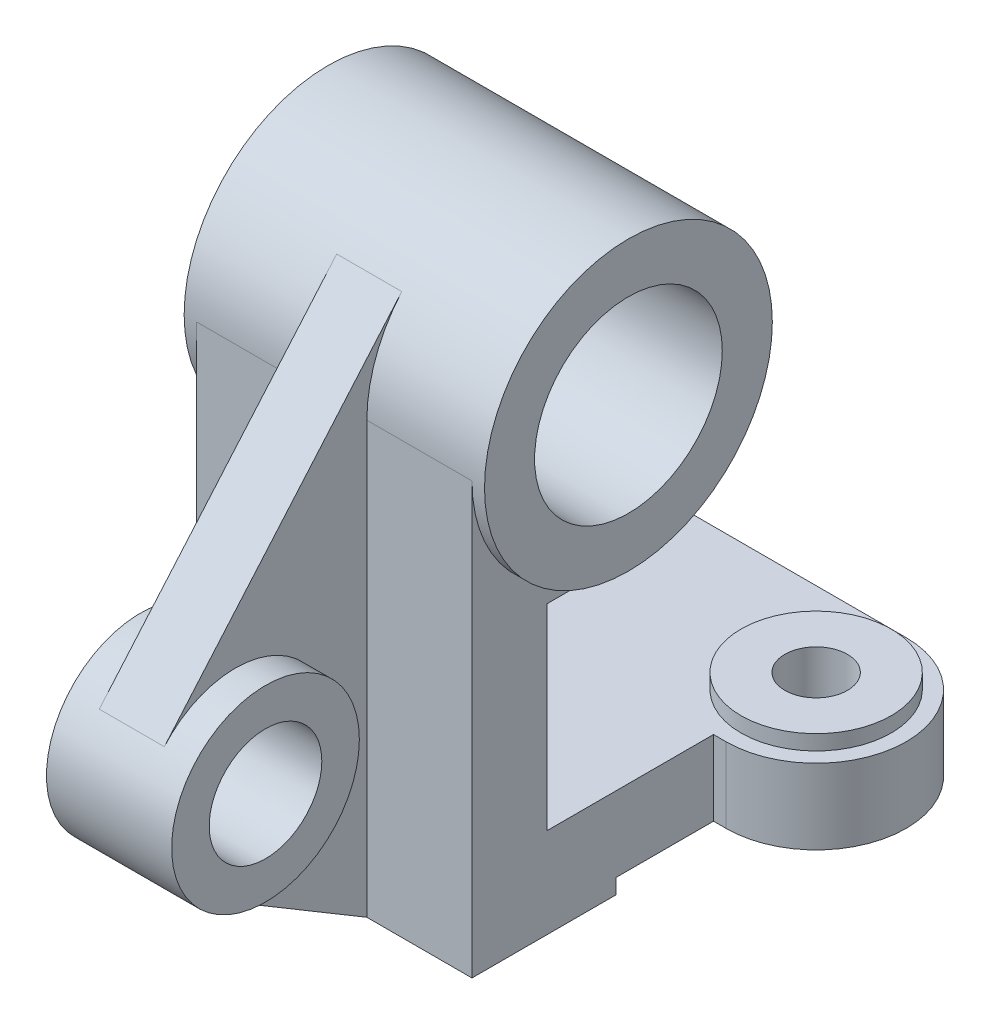
ISO-10303-21;
HEADER;
FILE_DESCRIPTION(('STEP AP214'),'2;1');
FILE_NAME('part.step','',(''),(''),'','','');
FILE_SCHEMA(('AUTOMOTIVE_DESIGN { 1 0 10303 214 1 1 1 1 }'));
ENDSEC;
DATA;
#1=APPLICATION_CONTEXT('core data for automotive mechanical design processes');
#2=APPLICATION_PROTOCOL_DEFINITION('international standard','automotive_design',2000,#1);
#3=PRODUCT_CONTEXT('',#1,'mechanical');
#4=PRODUCT('Part','Part','',(#3));
#5=PRODUCT_RELATED_PRODUCT_CATEGORY('part','',(#4));
#6=PRODUCT_DEFINITION_FORMATION('','',#4);
#7=PRODUCT_DEFINITION_CONTEXT('part definition',#1,'design');
#8=PRODUCT_DEFINITION('design','',#6,#7);
#9=PRODUCT_DEFINITION_SHAPE('','',#8);
#10=(LENGTH_UNIT() NAMED_UNIT(*) SI_UNIT(.MILLI.,.METRE.));
#11=(NAMED_UNIT(*) PLANE_ANGLE_UNIT() SI_UNIT($,.RADIAN.));
#12=(NAMED_UNIT(*) SI_UNIT($,.STERADIAN.) SOLID_ANGLE_UNIT());
#13=UNCERTAINTY_MEASURE_WITH_UNIT(LENGTH_MEASURE(1.E-05),#10,'distance_accuracy_value','');
#14=(GEOMETRIC_REPRESENTATION_CONTEXT(3) GLOBAL_UNCERTAINTY_ASSIGNED_CONTEXT((#13)) GLOBAL_UNIT_ASSIGNED_CONTEXT((#10,
#11,#12)) REPRESENTATION_CONTEXT('',''));
#15=CARTESIAN_POINT('',(0.,0.,0.));
#16=DIRECTION('',(0.,0.,1.));
#17=DIRECTION('',(1.,0.,0.));
#18=AXIS2_PLACEMENT_3D('',#15,#16,#17);
#19=CARTESIAN_POINT('',(55.,0.,57.5));
#20=DIRECTION('',(0.,0.,-1.));
#21=DIRECTION('',(0.,1.,0.));
#22=AXIS2_PLACEMENT_3D('',#19,#20,#21);
#23=PLANE('',#22);
#24=DIRECTION('',(0.,1.,0.));
#25=VECTOR('',#24,1.);
#26=CARTESIAN_POINT('',(-13.,-172.,57.5));
#27=LINE('',#26,#25);
#28=CARTESIAN_POINT('',(-13.,-172.,57.5));
#29=VERTEX_POINT('',#28);
#30=CARTESIAN_POINT('',(-13.,0.,57.5));
#31=VERTEX_POINT('',#30);
#32=EDGE_CURVE('E53',#29,#31,#27,.T.);
#33=ORIENTED_EDGE('',*,*,#32,.T.);
#34=DIRECTION('',(-1.,0.,0.));
#35=VECTOR('',#34,1.);
#36=CARTESIAN_POINT('',(55.,0.,57.5));
#37=LINE('',#36,#35);
#38=CARTESIAN_POINT('',(-55.,0.,57.5));
#39=VERTEX_POINT('',#38);
#40=EDGE_CURVE('E61',#31,#39,#37,.T.);
#41=ORIENTED_EDGE('',*,*,#40,.T.);
#42=DIRECTION('',(0.,-1.,0.));
#43=VECTOR('',#42,1.);
#44=CARTESIAN_POINT('',(-55.,0.,57.5));
#45=LINE('',#44,#43);
#46=CARTESIAN_POINT('',(-55.,-172.,57.5));
#47=VERTEX_POINT('',#46);
#48=EDGE_CURVE('E287',#39,#47,#45,.T.);
#49=ORIENTED_EDGE('',*,*,#48,.T.);
#50=DIRECTION('',(-1.,0.,0.));
#51=VECTOR('',#50,1.);
#52=CARTESIAN_POINT('',(55.,-172.,57.5));
#53=LINE('',#52,#51);
#54=EDGE_CURVE('E319',#29,#47,#53,.T.);
#55=ORIENTED_EDGE('',*,*,#54,.F.);
#56=EDGE_LOOP('',(#33,#41,#49,#55));
#57=FACE_BOUND('',#56,.T.);
#58=ADVANCED_FACE('F39',(#57),#23,.F.);
#59=CARTESIAN_POINT('',(-60.,0.,0.));
#60=DIRECTION('',(1.,0.,0.));
#61=DIRECTION('',(0.,0.,-1.));
#62=AXIS2_PLACEMENT_3D('',#59,#60,#61);
#63=CYLINDRICAL_SURFACE('',#62,57.5);
#64=CARTESIAN_POINT('',(13.,0.,0.));
#65=DIRECTION('',(-1.,0.,0.));
#66=DIRECTION('',(0.,0.,-1.));
#67=AXIS2_PLACEMENT_3D('',#64,#65,#66);
#68=CIRCLE('',#67,57.5);
#69=CARTESIAN_POINT('',(13.,0.,57.5));
#70=VERTEX_POINT('',#69);
#71=CARTESIAN_POINT('',(13.,37.5380186304021,43.5562527922637));
#72=VERTEX_POINT('',#71);
#73=EDGE_CURVE('E360',#70,#72,#68,.T.);
#74=ORIENTED_EDGE('',*,*,#73,.F.);
#75=CARTESIAN_POINT('',(55.,0.,57.5));
#76=VERTEX_POINT('',#75);
#77=EDGE_CURVE('E322',#76,#70,#37,.T.);
#78=ORIENTED_EDGE('',*,*,#77,.F.);
#79=CARTESIAN_POINT('',(55.,0.,0.));
#80=DIRECTION('',(-1.,0.,0.));
#81=DIRECTION('',(0.,0.,-1.));
#82=AXIS2_PLACEMENT_3D('',#79,#80,#81);
#83=CIRCLE('',#82,57.5);
#84=CARTESIAN_POINT('',(55.,-57.5,0.));
#85=VERTEX_POINT('',#84);
#86=EDGE_CURVE('E270',#85,#76,#83,.T.);
#87=ORIENTED_EDGE('',*,*,#86,.F.);
#88=DIRECTION('',(-1.,0.,0.));
#89=VECTOR('',#88,1.);
#90=CARTESIAN_POINT('',(55.,-57.5,0.));
#91=LINE('',#90,#89);
#92=CARTESIAN_POINT('',(-55.,-57.5,0.));
#93=VERTEX_POINT('',#92);
#94=EDGE_CURVE('E286',#85,#93,#91,.T.);
#95=ORIENTED_EDGE('',*,*,#94,.T.);
#96=CARTESIAN_POINT('',(-55.,0.,0.));
#97=DIRECTION('',(-1.,0.,0.));
#98=DIRECTION('',(0.,0.,-1.));
#99=AXIS2_PLACEMENT_3D('',#96,#97,#98);
#100=CIRCLE('',#99,57.5);
#101=EDGE_CURVE('E227',#93,#39,#100,.T.);
#102=ORIENTED_EDGE('',*,*,#101,.T.);
#103=ORIENTED_EDGE('',*,*,#40,.F.);
#104=CARTESIAN_POINT('',(-13.,0.,0.));
#105=DIRECTION('',(-1.,0.,0.));
#106=DIRECTION('',(0.,0.,-1.));
#107=AXIS2_PLACEMENT_3D('',#104,#105,#106);
#108=CIRCLE('',#107,57.5);
#109=CARTESIAN_POINT('',(-13.,37.5380186304021,43.5562527922637));
#110=VERTEX_POINT('',#109);
#111=EDGE_CURVE('E196',#31,#110,#108,.T.);
#112=ORIENTED_EDGE('',*,*,#111,.T.);
#113=DIRECTION('',(-1.,0.,0.));
#114=VECTOR('',#113,1.);
#115=CARTESIAN_POINT('',(13.,37.5380186304021,43.5562527922637));
#116=LINE('',#115,#114);
#117=EDGE_CURVE('E202',#72,#110,#116,.T.);
#118=ORIENTED_EDGE('',*,*,#117,.F.);
#119=EDGE_LOOP('',(#74,#78,#87,#95,#102,#103,#112,#118));
#120=FACE_BOUND('',#119,.T.);
#121=CARTESIAN_POINT('',(-60.,0.,0.));
#122=DIRECTION('',(1.,0.,0.));
#123=DIRECTION('',(0.,0.,-1.));
#124=AXIS2_PLACEMENT_3D('',#121,#122,#123);
#125=CIRCLE('',#124,57.5);
#126=CARTESIAN_POINT('',(-60.,0.,-57.5));
#127=VERTEX_POINT('',#126);
#128=EDGE_CURVE('E11',#127,#127,#125,.T.);
#129=ORIENTED_EDGE('',*,*,#128,.T.);
#130=EDGE_LOOP('',(#129));
#131=FACE_BOUND('',#130,.T.);
#132=CARTESIAN_POINT('',(60.,0.,0.));
#133=DIRECTION('',(1.,0.,0.));
#134=DIRECTION('',(0.,0.,-1.));
#135=AXIS2_PLACEMENT_3D('',#132,#133,#134);
#136=CIRCLE('',#135,57.5);
#137=CARTESIAN_POINT('',(60.,0.,-57.5));
#138=VERTEX_POINT('',#137);
#139=EDGE_CURVE('E43',#138,#138,#136,.T.);
#140=ORIENTED_EDGE('',*,*,#139,.F.);
#141=EDGE_LOOP('',(#140));
#142=FACE_BOUND('',#141,.T.);
#143=ADVANCED_FACE('F41',(#120,#131,#142),#63,.T.);
#144=CARTESIAN_POINT('',(-60.,0.,0.));
#145=DIRECTION('',(1.,0.,0.));
#146=DIRECTION('',(0.,0.,-1.));
#147=AXIS2_PLACEMENT_3D('',#144,#145,#146);
#148=PLANE('',#147);
#149=CARTESIAN_POINT('',(-60.,0.,0.));
#150=DIRECTION('',(1.,0.,0.));
#151=DIRECTION('',(0.,0.,-1.));
#152=AXIS2_PLACEMENT_3D('',#149,#150,#151);
#153=CIRCLE('',#152,37.5);
#154=CARTESIAN_POINT('',(-60.,0.,-37.5));
#155=VERTEX_POINT('',#154);
#156=EDGE_CURVE('E327',#155,#155,#153,.T.);
#157=ORIENTED_EDGE('',*,*,#156,.T.);
#158=EDGE_LOOP('',(#157));
#159=FACE_BOUND('',#158,.T.);
#160=ORIENTED_EDGE('',*,*,#128,.F.);
#161=EDGE_LOOP('',(#160));
#162=FACE_BOUND('',#161,.T.);
#163=ADVANCED_FACE('F338',(#159,#162),#148,.F.);
#164=CARTESIAN_POINT('',(60.,0.,0.));
#165=DIRECTION('',(1.,0.,0.));
#166=DIRECTION('',(0.,0.,-1.));
#167=AXIS2_PLACEMENT_3D('',#164,#165,#166);
#168=PLANE('',#167);
#169=CARTESIAN_POINT('',(60.,0.,0.));
#170=DIRECTION('',(1.,0.,0.));
#171=DIRECTION('',(0.,0.,-1.));
#172=AXIS2_PLACEMENT_3D('',#169,#170,#171);
#173=CIRCLE('',#172,37.5);
#174=CARTESIAN_POINT('',(60.,0.,-37.5));
#175=VERTEX_POINT('',#174);
#176=EDGE_CURVE('E330',#175,#175,#173,.T.);
#177=ORIENTED_EDGE('',*,*,#176,.F.);
#178=EDGE_LOOP('',(#177));
#179=FACE_BOUND('',#178,.T.);
#180=ORIENTED_EDGE('',*,*,#139,.T.);
#181=EDGE_LOOP('',(#180));
#182=FACE_BOUND('',#181,.T.);
#183=ADVANCED_FACE('F336',(#179,#182),#168,.T.);
#184=CARTESIAN_POINT('',(-60.,0.,0.));
#185=DIRECTION('',(1.,0.,0.));
#186=DIRECTION('',(0.,0.,-1.));
#187=AXIS2_PLACEMENT_3D('',#184,#185,#186);
#188=CYLINDRICAL_SURFACE('',#187,37.5);
#189=CARTESIAN_POINT('',(-60.,0.,-37.5));
#190=CARTESIAN_POINT('',(-58.75,0.,-37.5));
#191=CARTESIAN_POINT('',(-57.5,0.,-37.5));
#192=CARTESIAN_POINT('',(-55.,0.,-37.5));
#193=CARTESIAN_POINT('',(-53.75,0.,-37.5));
#194=CARTESIAN_POINT('',(-51.25,0.,-37.5));
#195=CARTESIAN_POINT('',(-50.,0.,-37.5));
#196=CARTESIAN_POINT('',(-47.5,0.,-37.5));
#197=CARTESIAN_POINT('',(-46.25,0.,-37.5));
#198=CARTESIAN_POINT('',(-43.75,0.,-37.5));
#199=CARTESIAN_POINT('',(-42.5,0.,-37.5));
#200=CARTESIAN_POINT('',(-40.,0.,-37.5));
#201=CARTESIAN_POINT('',(-38.75,0.,-37.5));
#202=CARTESIAN_POINT('',(-36.25,0.,-37.5));
#203=CARTESIAN_POINT('',(-35.,0.,-37.5));
#204=CARTESIAN_POINT('',(-32.5,0.,-37.5));
#205=CARTESIAN_POINT('',(-31.25,0.,-37.5));
#206=CARTESIAN_POINT('',(-28.75,0.,-37.5));
#207=CARTESIAN_POINT('',(-27.5,0.,-37.5));
#208=CARTESIAN_POINT('',(-25.,0.,-37.5));
#209=CARTESIAN_POINT('',(-23.75,0.,-37.5));
#210=CARTESIAN_POINT('',(-21.25,0.,-37.5));
#211=CARTESIAN_POINT('',(-20.,0.,-37.5));
#212=CARTESIAN_POINT('',(-17.5,0.,-37.5));
#213=CARTESIAN_POINT('',(-16.25,0.,-37.5));
#214=CARTESIAN_POINT('',(-13.75,0.,-37.5));
#215=CARTESIAN_POINT('',(-12.5,0.,-37.5));
#216=CARTESIAN_POINT('',(-10.,0.,-37.5));
#217=CARTESIAN_POINT('',(-8.75000000000001,0.,-37.5));
#218=CARTESIAN_POINT('',(-6.25000000000001,0.,-37.5));
#219=CARTESIAN_POINT('',(-5.00000000000001,0.,-37.5));
#220=CARTESIAN_POINT('',(-2.50000000000001,0.,-37.5));
#221=CARTESIAN_POINT('',(-1.25000000000001,0.,-37.5));
#222=CARTESIAN_POINT('',(1.24999999999999,0.,-37.5));
#223=CARTESIAN_POINT('',(2.5,0.,-37.5));
#224=CARTESIAN_POINT('',(5.,0.,-37.5));
#225=CARTESIAN_POINT('',(6.25,0.,-37.5));
#226=CARTESIAN_POINT('',(8.75,0.,-37.5));
#227=CARTESIAN_POINT('',(9.99999999999999,0.,-37.5));
#228=CARTESIAN_POINT('',(12.5,0.,-37.5));
#229=CARTESIAN_POINT('',(13.75,0.,-37.5));
#230=CARTESIAN_POINT('',(16.25,0.,-37.5));
#231=CARTESIAN_POINT('',(17.5,0.,-37.5));
#232=CARTESIAN_POINT('',(20.,0.,-37.5));
#233=CARTESIAN_POINT('',(21.25,0.,-37.5));
#234=CARTESIAN_POINT('',(23.75,0.,-37.5));
#235=CARTESIAN_POINT('',(25.,0.,-37.5));
#236=CARTESIAN_POINT('',(27.5,0.,-37.5));
#237=CARTESIAN_POINT('',(28.75,0.,-37.5));
#238=CARTESIAN_POINT('',(31.25,0.,-37.5));
#239=CARTESIAN_POINT('',(32.5,0.,-37.5));
#240=CARTESIAN_POINT('',(35.,0.,-37.5));
#241=CARTESIAN_POINT('',(36.25,0.,-37.5));
#242=CARTESIAN_POINT('',(38.75,0.,-37.5));
#243=CARTESIAN_POINT('',(40.,0.,-37.5));
#244=CARTESIAN_POINT('',(42.5,0.,-37.5));
#245=CARTESIAN_POINT('',(43.75,0.,-37.5));
#246=CARTESIAN_POINT('',(46.25,0.,-37.5));
#247=CARTESIAN_POINT('',(47.5,0.,-37.5));
#248=CARTESIAN_POINT('',(50.,0.,-37.5));
#249=CARTESIAN_POINT('',(51.25,0.,-37.5));
#250=CARTESIAN_POINT('',(53.75,0.,-37.5));
#251=CARTESIAN_POINT('',(55.,0.,-37.5));
#252=CARTESIAN_POINT('',(57.5,0.,-37.5));
#253=CARTESIAN_POINT('',(58.75,0.,-37.5));
#254=CARTESIAN_POINT('',(60.,0.,-37.5));
#255=B_SPLINE_CURVE_WITH_KNOTS('',3,(#189,#190,#191,#192,#193,#194,#195,#196,#197,#198,#199,
#200,#201,#202,#203,#204,#205,#206,#207,#208,#209,#210,#211,#212,#213,#214,#215,#216,#217,#218,
#219,#220,#221,#222,#223,#224,#225,#226,#227,#228,#229,#230,#231,#232,#233,#234,#235,#236,#237,
#238,#239,#240,#241,#242,#243,#244,#245,#246,#247,#248,#249,#250,#251,#252,#253,#254),
.UNSPECIFIED.,.F.,.F.,(4,2,2,2,2,2,2,2,2,2,2,2,2,2,2,2,2,2,2,2,2,2,2,2,2,2,2,2,2,2,2,2,4),(0.,
3.75,7.5,11.25,15.,18.75,22.5,26.25,30.,33.75,37.5,41.25,45.,48.75,52.5,56.25,60.,63.75,67.5,
71.25,75.,78.75,82.5,86.25,90.,93.75,97.5,101.25,105.,108.75,112.5,116.25,120.),.UNSPECIFIED.);
#256=EDGE_CURVE('BSEAM331',#155,#175,#255,.T.);
#257=ORIENTED_EDGE('',*,*,#156,.F.);
#258=ORIENTED_EDGE('',*,*,#176,.T.);
#259=ORIENTED_EDGE('',*,*,#256,.T.);
#260=ORIENTED_EDGE('',*,*,#256,.F.);
#261=EDGE_LOOP('',(#257,#259,#258,#260));
#262=FACE_BOUND('',#261,.T.);
#263=ADVANCED_FACE('F331',(#262),#188,.F.);
#264=ORIENTED_EDGE('',*,*,#77,.T.);
#265=DIRECTION('',(0.,1.,0.));
#266=VECTOR('',#265,1.);
#267=CARTESIAN_POINT('',(13.,-172.,57.5));
#268=LINE('',#267,#266);
#269=CARTESIAN_POINT('',(13.,-172.,57.5));
#270=VERTEX_POINT('',#269);
#271=EDGE_CURVE('E365',#270,#70,#268,.T.);
#272=ORIENTED_EDGE('',*,*,#271,.F.);
#273=CARTESIAN_POINT('',(55.,-172.,57.5));
#274=VERTEX_POINT('',#273);
#275=EDGE_CURVE('E321',#274,#270,#53,.T.);
#276=ORIENTED_EDGE('',*,*,#275,.F.);
#277=DIRECTION('',(0.,-1.,0.));
#278=VECTOR('',#277,1.);
#279=CARTESIAN_POINT('',(55.,0.,57.5));
#280=LINE('',#279,#278);
#281=EDGE_CURVE('E269',#76,#274,#280,.T.);
#282=ORIENTED_EDGE('',*,*,#281,.F.);
#283=EDGE_LOOP('',(#264,#272,#276,#282));
#284=FACE_BOUND('',#283,.T.);
#285=ADVANCED_FACE('F354',(#284),#23,.F.);
#286=CARTESIAN_POINT('',(55.,-172.,57.5));
#287=DIRECTION('',(0.,1.,0.));
#288=DIRECTION('',(0.,0.,1.));
#289=AXIS2_PLACEMENT_3D('',#286,#287,#288);
#290=PLANE('',#289);
#291=DIRECTION('',(0.,0.,-1.));
#292=VECTOR('',#291,1.);
#293=CARTESIAN_POINT('',(-55.,-172.,57.5));
#294=LINE('',#293,#292);
#295=CARTESIAN_POINT('',(-55.,-172.,0.));
#296=VERTEX_POINT('',#295);
#297=EDGE_CURVE('E295',#47,#296,#294,.T.);
#298=ORIENTED_EDGE('',*,*,#297,.T.);
#299=DIRECTION('',(-1.,0.,0.));
#300=VECTOR('',#299,1.);
#301=CARTESIAN_POINT('',(55.,-172.,0.));
#302=LINE('',#301,#300);
#303=CARTESIAN_POINT('',(55.,-172.,0.));
#304=VERTEX_POINT('',#303);
#305=EDGE_CURVE('E320',#304,#296,#302,.T.);
#306=ORIENTED_EDGE('',*,*,#305,.F.);
#307=DIRECTION('',(0.,0.,-1.));
#308=VECTOR('',#307,1.);
#309=CARTESIAN_POINT('',(55.,-172.,57.5));
#310=LINE('',#309,#308);
#311=EDGE_CURVE('E272',#274,#304,#310,.T.);
#312=ORIENTED_EDGE('',*,*,#311,.F.);
#313=ORIENTED_EDGE('',*,*,#275,.T.);
#314=DIRECTION('',(-1.,0.,0.));
#315=VECTOR('',#314,1.);
#316=CARTESIAN_POINT('',(13.,-172.,57.5));
#317=LINE('',#316,#315);
#318=EDGE_CURVE('E179',#270,#29,#317,.T.);
#319=ORIENTED_EDGE('',*,*,#318,.T.);
#320=ORIENTED_EDGE('',*,*,#54,.T.);
#321=EDGE_LOOP('',(#298,#306,#312,#313,#319,#320));
#322=FACE_BOUND('',#321,.T.);
#323=ADVANCED_FACE('F383',(#322),#290,.F.);
#324=CARTESIAN_POINT('',(55.,-172.,0.));
#325=DIRECTION('',(0.,0.,1.));
#326=DIRECTION('',(0.,-1.,0.));
#327=AXIS2_PLACEMENT_3D('',#324,#325,#326);
#328=PLANE('',#327);
#329=DIRECTION('',(0.,1.,0.));
#330=VECTOR('',#329,1.);
#331=CARTESIAN_POINT('',(-55.,-172.,0.));
#332=LINE('',#331,#330);
#333=CARTESIAN_POINT('',(-55.,-166.,0.));
#334=VERTEX_POINT('',#333);
#335=EDGE_CURVE('E294',#296,#334,#332,.T.);
#336=ORIENTED_EDGE('',*,*,#335,.T.);
#337=DIRECTION('',(-1.,0.,0.));
#338=VECTOR('',#337,1.);
#339=CARTESIAN_POINT('',(55.,-166.,0.));
#340=LINE('',#339,#338);
#341=CARTESIAN_POINT('',(55.,-166.,0.));
#342=VERTEX_POINT('',#341);
#343=EDGE_CURVE('E314',#342,#334,#340,.T.);
#344=ORIENTED_EDGE('',*,*,#343,.F.);
#345=DIRECTION('',(0.,1.,0.));
#346=VECTOR('',#345,1.);
#347=CARTESIAN_POINT('',(55.,-172.,0.));
#348=LINE('',#347,#346);
#349=EDGE_CURVE('E274',#304,#342,#348,.T.);
#350=ORIENTED_EDGE('',*,*,#349,.F.);
#351=ORIENTED_EDGE('',*,*,#305,.T.);
#352=EDGE_LOOP('',(#336,#344,#350,#351));
#353=FACE_BOUND('',#352,.T.);
#354=ADVANCED_FACE('F391',(#353),#328,.F.);
#355=CARTESIAN_POINT('',(55.,-166.,0.));
#356=DIRECTION('',(0.,1.,0.));
#357=DIRECTION('',(0.,0.,1.));
#358=AXIS2_PLACEMENT_3D('',#355,#356,#357);
#359=PLANE('',#358);
#360=DIRECTION('',(0.,0.,-1.));
#361=VECTOR('',#360,1.);
#362=CARTESIAN_POINT('',(-55.,-166.,0.));
#363=LINE('',#362,#361);
#364=CARTESIAN_POINT('',(-55.,-166.,-39.));
#365=VERTEX_POINT('',#364);
#366=EDGE_CURVE('E296',#334,#365,#363,.T.);
#367=ORIENTED_EDGE('',*,*,#366,.T.);
#368=DIRECTION('',(1.,0.,0.));
#369=VECTOR('',#368,1.);
#370=CARTESIAN_POINT('',(-60.,-166.,-39.));
#371=LINE('',#370,#369);
#372=CARTESIAN_POINT('',(-60.,-166.,-39.));
#373=VERTEX_POINT('',#372);
#374=EDGE_CURVE('E253',#373,#365,#371,.T.);
#375=ORIENTED_EDGE('',*,*,#374,.F.);
#376=CARTESIAN_POINT('',(-60.,-166.,-75.));
#377=DIRECTION('',(0.,1.,0.));
#378=DIRECTION('',(0.,0.,1.));
#379=AXIS2_PLACEMENT_3D('',#376,#377,#378);
#380=CIRCLE('',#379,36.);
#381=CARTESIAN_POINT('',(-60.,-166.,-111.));
#382=VERTEX_POINT('',#381);
#383=EDGE_CURVE('E233',#382,#373,#380,.T.);
#384=ORIENTED_EDGE('',*,*,#383,.F.);
#385=DIRECTION('',(-1.,0.,0.));
#386=VECTOR('',#385,1.);
#387=CARTESIAN_POINT('',(-60.,-166.,-111.));
#388=LINE('',#387,#386);
#389=CARTESIAN_POINT('',(60.,-166.,-111.));
#390=VERTEX_POINT('',#389);
#391=EDGE_CURVE('E239',#390,#382,#388,.T.);
#392=ORIENTED_EDGE('',*,*,#391,.F.);
#393=CARTESIAN_POINT('',(60.,-166.,-75.));
#394=DIRECTION('',(0.,1.,0.));
#395=DIRECTION('',(0.,0.,1.));
#396=AXIS2_PLACEMENT_3D('',#393,#394,#395);
#397=CIRCLE('',#396,36.);
#398=CARTESIAN_POINT('',(60.,-166.,-39.));
#399=VERTEX_POINT('',#398);
#400=EDGE_CURVE('E255',#399,#390,#397,.T.);
#401=ORIENTED_EDGE('',*,*,#400,.F.);
#402=CARTESIAN_POINT('',(55.,-166.,-39.));
#403=VERTEX_POINT('',#402);
#404=EDGE_CURVE('E247',#403,#399,#371,.T.);
#405=ORIENTED_EDGE('',*,*,#404,.F.);
#406=DIRECTION('',(0.,0.,-1.));
#407=VECTOR('',#406,1.);
#408=CARTESIAN_POINT('',(55.,-166.,0.));
#409=LINE('',#408,#407);
#410=EDGE_CURVE('E280',#342,#403,#409,.T.);
#411=ORIENTED_EDGE('',*,*,#410,.F.);
#412=ORIENTED_EDGE('',*,*,#343,.T.);
#413=EDGE_LOOP('',(#367,#375,#384,#392,#401,#405,#411,#412));
#414=FACE_BOUND('',#413,.T.);
#415=CARTESIAN_POINT('',(60.,-166.,-75.));
#416=DIRECTION('',(0.,1.,0.));
#417=DIRECTION('',(0.,0.,1.));
#418=AXIS2_PLACEMENT_3D('',#415,#416,#417);
#419=CIRCLE('',#418,12.5);
#420=CARTESIAN_POINT('',(60.,-166.,-62.5));
#421=VERTEX_POINT('',#420);
#422=EDGE_CURVE('E234',#421,#421,#419,.T.);
#423=ORIENTED_EDGE('',*,*,#422,.T.);
#424=EDGE_LOOP('',(#423));
#425=FACE_BOUND('',#424,.T.);
#426=CARTESIAN_POINT('',(-60.,-166.,-75.));
#427=DIRECTION('',(0.,1.,0.));
#428=DIRECTION('',(0.,0.,1.));
#429=AXIS2_PLACEMENT_3D('',#426,#427,#428);
#430=CIRCLE('',#429,12.5);
#431=CARTESIAN_POINT('',(-60.,-166.,-62.5));
#432=VERTEX_POINT('',#431);
#433=EDGE_CURVE('E224',#432,#432,#430,.T.);
#434=ORIENTED_EDGE('',*,*,#433,.T.);
#435=EDGE_LOOP('',(#434));
#436=FACE_BOUND('',#435,.T.);
#437=ADVANCED_FACE('F395',(#414,#425,#436),#359,.F.);
#438=CARTESIAN_POINT('',(55.,-136.,27.5));
#439=DIRECTION('',(0.,-1.,0.));
#440=DIRECTION('',(0.,0.,-1.));
#441=AXIS2_PLACEMENT_3D('',#438,#439,#440);
#442=PLANE('',#441);
#443=DIRECTION('',(0.,0.,1.));
#444=VECTOR('',#443,1.);
#445=CARTESIAN_POINT('',(-55.,-136.,27.5));
#446=LINE('',#445,#444);
#447=CARTESIAN_POINT('',(-55.,-136.,-39.));
#448=VERTEX_POINT('',#447);
#449=CARTESIAN_POINT('',(-55.,-136.,27.5));
#450=VERTEX_POINT('',#449);
#451=EDGE_CURVE('E304',#448,#450,#446,.T.);
#452=ORIENTED_EDGE('',*,*,#451,.T.);
#453=DIRECTION('',(-1.,0.,0.));
#454=VECTOR('',#453,1.);
#455=CARTESIAN_POINT('',(55.,-136.,27.5));
#456=LINE('',#455,#454);
#457=CARTESIAN_POINT('',(55.,-136.,27.5));
#458=VERTEX_POINT('',#457);
#459=EDGE_CURVE('E313',#458,#450,#456,.T.);
#460=ORIENTED_EDGE('',*,*,#459,.F.);
#461=DIRECTION('',(0.,0.,1.));
#462=VECTOR('',#461,1.);
#463=CARTESIAN_POINT('',(55.,-136.,27.5));
#464=LINE('',#463,#462);
#465=CARTESIAN_POINT('',(55.,-136.,-39.));
#466=VERTEX_POINT('',#465);
#467=EDGE_CURVE('E281',#466,#458,#464,.T.);
#468=ORIENTED_EDGE('',*,*,#467,.F.);
#469=DIRECTION('',(1.,0.,0.));
#470=VECTOR('',#469,1.);
#471=CARTESIAN_POINT('',(-60.,-136.,-39.));
#472=LINE('',#471,#470);
#473=CARTESIAN_POINT('',(60.,-136.,-39.));
#474=VERTEX_POINT('',#473);
#475=EDGE_CURVE('E236',#466,#474,#472,.T.);
#476=ORIENTED_EDGE('',*,*,#475,.T.);
#477=CARTESIAN_POINT('',(60.,-136.,-75.));
#478=DIRECTION('',(0.,1.,0.));
#479=DIRECTION('',(0.,0.,1.));
#480=AXIS2_PLACEMENT_3D('',#477,#478,#479);
#481=CIRCLE('',#480,36.);
#482=CARTESIAN_POINT('',(60.,-136.,-111.));
#483=VERTEX_POINT('',#482);
#484=EDGE_CURVE('E244',#474,#483,#481,.T.);
#485=ORIENTED_EDGE('',*,*,#484,.T.);
#486=DIRECTION('',(-1.,0.,0.));
#487=VECTOR('',#486,1.);
#488=CARTESIAN_POINT('',(-60.,-136.,-111.));
#489=LINE('',#488,#487);
#490=CARTESIAN_POINT('',(-60.,-136.,-111.));
#491=VERTEX_POINT('',#490);
#492=EDGE_CURVE('E245',#483,#491,#489,.T.);
#493=ORIENTED_EDGE('',*,*,#492,.T.);
#494=CARTESIAN_POINT('',(-60.,-136.,-75.));
#495=DIRECTION('',(0.,1.,0.));
#496=DIRECTION('',(0.,0.,1.));
#497=AXIS2_PLACEMENT_3D('',#494,#495,#496);
#498=CIRCLE('',#497,36.);
#499=CARTESIAN_POINT('',(-60.,-136.,-39.));
#500=VERTEX_POINT('',#499);
#501=EDGE_CURVE('E232',#491,#500,#498,.T.);
#502=ORIENTED_EDGE('',*,*,#501,.T.);
#503=EDGE_CURVE('E238',#500,#448,#472,.T.);
#504=ORIENTED_EDGE('',*,*,#503,.T.);
#505=EDGE_LOOP('',(#452,#460,#468,#476,#485,#493,#502,#504));
#506=FACE_BOUND('',#505,.T.);
#507=CARTESIAN_POINT('',(60.,-136.,-75.));
#508=DIRECTION('',(0.,1.,0.));
#509=DIRECTION('',(0.,0.,1.));
#510=AXIS2_PLACEMENT_3D('',#507,#508,#509);
#511=CIRCLE('',#510,30.);
#512=CARTESIAN_POINT('',(60.,-136.,-45.));
#513=VERTEX_POINT('',#512);
#514=EDGE_CURVE('E221',#513,#513,#511,.T.);
#515=ORIENTED_EDGE('',*,*,#514,.F.);
#516=EDGE_LOOP('',(#515));
#517=FACE_BOUND('',#516,.T.);
#518=CARTESIAN_POINT('',(-60.,-136.,-75.));
#519=DIRECTION('',(0.,1.,0.));
#520=DIRECTION('',(0.,0.,1.));
#521=AXIS2_PLACEMENT_3D('',#518,#519,#520);
#522=CIRCLE('',#521,30.);
#523=CARTESIAN_POINT('',(-60.,-136.,-45.));
#524=VERTEX_POINT('',#523);
#525=EDGE_CURVE('E211',#524,#524,#522,.T.);
#526=ORIENTED_EDGE('',*,*,#525,.F.);
#527=EDGE_LOOP('',(#526));
#528=FACE_BOUND('',#527,.T.);
#529=ADVANCED_FACE('F408',(#506,#517,#528),#442,.F.);
#530=CARTESIAN_POINT('',(55.,-57.5,27.5));
#531=DIRECTION('',(0.,0.,1.));
#532=DIRECTION('',(0.,-1.,0.));
#533=AXIS2_PLACEMENT_3D('',#530,#531,#532);
#534=PLANE('',#533);
#535=DIRECTION('',(0.,1.,0.));
#536=VECTOR('',#535,1.);
#537=CARTESIAN_POINT('',(-55.,-57.5,27.5));
#538=LINE('',#537,#536);
#539=CARTESIAN_POINT('',(-55.,-57.5,27.5));
#540=VERTEX_POINT('',#539);
#541=EDGE_CURVE('E305',#450,#540,#538,.T.);
#542=ORIENTED_EDGE('',*,*,#541,.T.);
#543=DIRECTION('',(-1.,0.,0.));
#544=VECTOR('',#543,1.);
#545=CARTESIAN_POINT('',(55.,-57.5,27.5));
#546=LINE('',#545,#544);
#547=CARTESIAN_POINT('',(55.,-57.5,27.5));
#548=VERTEX_POINT('',#547);
#549=EDGE_CURVE('E306',#548,#540,#546,.T.);
#550=ORIENTED_EDGE('',*,*,#549,.F.);
#551=DIRECTION('',(0.,1.,0.));
#552=VECTOR('',#551,1.);
#553=CARTESIAN_POINT('',(55.,-57.5,27.5));
#554=LINE('',#553,#552);
#555=EDGE_CURVE('E284',#458,#548,#554,.T.);
#556=ORIENTED_EDGE('',*,*,#555,.F.);
#557=ORIENTED_EDGE('',*,*,#459,.T.);
#558=EDGE_LOOP('',(#542,#550,#556,#557));
#559=FACE_BOUND('',#558,.T.);
#560=ADVANCED_FACE('F418',(#559),#534,.F.);
#561=CARTESIAN_POINT('',(55.,-57.5,0.));
#562=DIRECTION('',(0.,1.,0.));
#563=DIRECTION('',(0.,0.,1.));
#564=AXIS2_PLACEMENT_3D('',#561,#562,#563);
#565=PLANE('',#564);
#566=DIRECTION('',(0.,0.,-1.));
#567=VECTOR('',#566,1.);
#568=CARTESIAN_POINT('',(-55.,-57.5,0.));
#569=LINE('',#568,#567);
#570=EDGE_CURVE('E271',#540,#93,#569,.T.);
#571=ORIENTED_EDGE('',*,*,#570,.T.);
#572=ORIENTED_EDGE('',*,*,#94,.F.);
#573=DIRECTION('',(0.,0.,-1.));
#574=VECTOR('',#573,1.);
#575=CARTESIAN_POINT('',(55.,-57.5,0.));
#576=LINE('',#575,#574);
#577=EDGE_CURVE('E285',#548,#85,#576,.T.);
#578=ORIENTED_EDGE('',*,*,#577,.F.);
#579=ORIENTED_EDGE('',*,*,#549,.T.);
#580=EDGE_LOOP('',(#571,#572,#578,#579));
#581=FACE_BOUND('',#580,.T.);
#582=ADVANCED_FACE('F374',(#581),#565,.F.);
#583=CARTESIAN_POINT('',(55.,0.,0.));
#584=DIRECTION('',(1.,0.,0.));
#585=DIRECTION('',(0.,0.,-1.));
#586=AXIS2_PLACEMENT_3D('',#583,#584,#585);
#587=PLANE('',#586);
#588=ORIENTED_EDGE('',*,*,#86,.T.);
#589=ORIENTED_EDGE('',*,*,#281,.T.);
#590=ORIENTED_EDGE('',*,*,#311,.T.);
#591=ORIENTED_EDGE('',*,*,#349,.T.);
#592=ORIENTED_EDGE('',*,*,#410,.T.);
#593=DIRECTION('',(0.,1.,0.));
#594=VECTOR('',#593,1.);
#595=CARTESIAN_POINT('',(55.,-136.,-39.));
#596=LINE('',#595,#594);
#597=EDGE_CURVE('E276',#403,#466,#596,.T.);
#598=ORIENTED_EDGE('',*,*,#597,.T.);
#599=ORIENTED_EDGE('',*,*,#467,.T.);
#600=ORIENTED_EDGE('',*,*,#555,.T.);
#601=ORIENTED_EDGE('',*,*,#577,.T.);
#602=EDGE_LOOP('',(#588,#589,#590,#591,#592,#598,#599,#600,#601));
#603=FACE_BOUND('',#602,.T.);
#604=ADVANCED_FACE('F367',(#603),#587,.T.);
#605=CARTESIAN_POINT('',(-55.,0.,0.));
#606=DIRECTION('',(1.,0.,0.));
#607=DIRECTION('',(0.,0.,-1.));
#608=AXIS2_PLACEMENT_3D('',#605,#606,#607);
#609=PLANE('',#608);
#610=ORIENTED_EDGE('',*,*,#101,.F.);
#611=ORIENTED_EDGE('',*,*,#570,.F.);
#612=ORIENTED_EDGE('',*,*,#541,.F.);
#613=ORIENTED_EDGE('',*,*,#451,.F.);
#614=DIRECTION('',(0.,1.,0.));
#615=VECTOR('',#614,1.);
#616=CARTESIAN_POINT('',(-55.,-136.,-39.));
#617=LINE('',#616,#615);
#618=EDGE_CURVE('E299',#365,#448,#617,.T.);
#619=ORIENTED_EDGE('',*,*,#618,.F.);
#620=ORIENTED_EDGE('',*,*,#366,.F.);
#621=ORIENTED_EDGE('',*,*,#335,.F.);
#622=ORIENTED_EDGE('',*,*,#297,.F.);
#623=ORIENTED_EDGE('',*,*,#48,.F.);
#624=EDGE_LOOP('',(#610,#611,#612,#613,#619,#620,#621,#622,#623));
#625=FACE_BOUND('',#624,.T.);
#626=ADVANCED_FACE('F379',(#625),#609,.F.);
#627=CARTESIAN_POINT('',(-60.,-136.,-39.));
#628=DIRECTION('',(0.,0.,-1.));
#629=DIRECTION('',(-1.,0.,0.));
#630=AXIS2_PLACEMENT_3D('',#627,#628,#629);
#631=PLANE('',#630);
#632=ORIENTED_EDGE('',*,*,#374,.T.);
#633=ORIENTED_EDGE('',*,*,#618,.T.);
#634=ORIENTED_EDGE('',*,*,#503,.F.);
#635=DIRECTION('',(0.,-1.,0.));
#636=VECTOR('',#635,1.);
#637=CARTESIAN_POINT('',(-60.,-136.,-39.));
#638=LINE('',#637,#636);
#639=EDGE_CURVE('E229',#500,#373,#638,.T.);
#640=ORIENTED_EDGE('',*,*,#639,.T.);
#641=EDGE_LOOP('',(#632,#633,#634,#640));
#642=FACE_BOUND('',#641,.T.);
#643=ADVANCED_FACE('F420',(#642),#631,.F.);
#644=CARTESIAN_POINT('',(-60.,-136.,-75.));
#645=DIRECTION('',(0.,-1.,0.));
#646=DIRECTION('',(0.,0.,-1.));
#647=AXIS2_PLACEMENT_3D('',#644,#645,#646);
#648=CYLINDRICAL_SURFACE('',#647,36.);
#649=ORIENTED_EDGE('',*,*,#383,.T.);
#650=ORIENTED_EDGE('',*,*,#639,.F.);
#651=ORIENTED_EDGE('',*,*,#501,.F.);
#652=DIRECTION('',(0.,-1.,0.));
#653=VECTOR('',#652,1.);
#654=CARTESIAN_POINT('',(-60.,-136.,-111.));
#655=LINE('',#654,#653);
#656=EDGE_CURVE('E246',#491,#382,#655,.T.);
#657=ORIENTED_EDGE('',*,*,#656,.T.);
#658=EDGE_LOOP('',(#649,#650,#651,#657));
#659=FACE_BOUND('',#658,.T.);
#660=ADVANCED_FACE('F421',(#659),#648,.T.);
#661=ORIENTED_EDGE('',*,*,#597,.F.);
#662=ORIENTED_EDGE('',*,*,#404,.T.);
#663=DIRECTION('',(0.,-1.,0.));
#664=VECTOR('',#663,1.);
#665=CARTESIAN_POINT('',(60.,-136.,-39.));
#666=LINE('',#665,#664);
#667=EDGE_CURVE('E265',#474,#399,#666,.T.);
#668=ORIENTED_EDGE('',*,*,#667,.F.);
#669=ORIENTED_EDGE('',*,*,#475,.F.);
#670=EDGE_LOOP('',(#661,#662,#668,#669));
#671=FACE_BOUND('',#670,.T.);
#672=ADVANCED_FACE('F402',(#671),#631,.F.);
#673=CARTESIAN_POINT('',(60.,-136.,-75.));
#674=DIRECTION('',(0.,-1.,0.));
#675=DIRECTION('',(0.,0.,-1.));
#676=AXIS2_PLACEMENT_3D('',#673,#674,#675);
#677=CYLINDRICAL_SURFACE('',#676,36.);
#678=ORIENTED_EDGE('',*,*,#400,.T.);
#679=DIRECTION('',(0.,-1.,0.));
#680=VECTOR('',#679,1.);
#681=CARTESIAN_POINT('',(60.,-136.,-111.));
#682=LINE('',#681,#680);
#683=EDGE_CURVE('E259',#483,#390,#682,.T.);
#684=ORIENTED_EDGE('',*,*,#683,.F.);
#685=ORIENTED_EDGE('',*,*,#484,.F.);
#686=ORIENTED_EDGE('',*,*,#667,.T.);
#687=EDGE_LOOP('',(#678,#684,#685,#686));
#688=FACE_BOUND('',#687,.T.);
#689=ADVANCED_FACE('F403',(#688),#677,.T.);
#690=CARTESIAN_POINT('',(-60.,-136.,-111.));
#691=DIRECTION('',(0.,0.,1.));
#692=DIRECTION('',(1.,0.,0.));
#693=AXIS2_PLACEMENT_3D('',#690,#691,#692);
#694=PLANE('',#693);
#695=ORIENTED_EDGE('',*,*,#391,.T.);
#696=ORIENTED_EDGE('',*,*,#656,.F.);
#697=ORIENTED_EDGE('',*,*,#492,.F.);
#698=ORIENTED_EDGE('',*,*,#683,.T.);
#699=EDGE_LOOP('',(#695,#696,#697,#698));
#700=FACE_BOUND('',#699,.T.);
#701=ADVANCED_FACE('F426',(#700),#694,.F.);
#702=CARTESIAN_POINT('',(60.,-136.,-75.));
#703=DIRECTION('',(0.,-1.,0.));
#704=DIRECTION('',(0.,0.,-1.));
#705=AXIS2_PLACEMENT_3D('',#702,#703,#704);
#706=CYLINDRICAL_SURFACE('',#705,12.5);
#707=ORIENTED_EDGE('',*,*,#422,.F.);
#708=EDGE_LOOP('',(#707));
#709=FACE_BOUND('',#708,.T.);
#710=CARTESIAN_POINT('',(60.,-130.,-75.));
#711=DIRECTION('',(0.,1.,0.));
#712=DIRECTION('',(0.,0.,1.));
#713=AXIS2_PLACEMENT_3D('',#710,#711,#712);
#714=CIRCLE('',#713,12.5);
#715=CARTESIAN_POINT('',(60.,-130.,-62.5));
#716=VERTEX_POINT('',#715);
#717=EDGE_CURVE('E214',#716,#716,#714,.T.);
#718=ORIENTED_EDGE('',*,*,#717,.T.);
#719=EDGE_LOOP('',(#718));
#720=FACE_BOUND('',#719,.T.);
#721=ADVANCED_FACE('F428',(#709,#720),#706,.F.);
#722=CARTESIAN_POINT('',(-60.,-136.,-75.));
#723=DIRECTION('',(0.,-1.,0.));
#724=DIRECTION('',(0.,0.,-1.));
#725=AXIS2_PLACEMENT_3D('',#722,#723,#724);
#726=CYLINDRICAL_SURFACE('',#725,12.5);
#727=ORIENTED_EDGE('',*,*,#433,.F.);
#728=EDGE_LOOP('',(#727));
#729=FACE_BOUND('',#728,.T.);
#730=CARTESIAN_POINT('',(-60.,-130.,-75.));
#731=DIRECTION('',(0.,1.,0.));
#732=DIRECTION('',(0.,0.,1.));
#733=AXIS2_PLACEMENT_3D('',#730,#731,#732);
#734=CIRCLE('',#733,12.5);
#735=CARTESIAN_POINT('',(-60.,-130.,-62.5));
#736=VERTEX_POINT('',#735);
#737=EDGE_CURVE('E175',#736,#736,#734,.T.);
#738=ORIENTED_EDGE('',*,*,#737,.T.);
#739=EDGE_LOOP('',(#738));
#740=FACE_BOUND('',#739,.T.);
#741=ADVANCED_FACE('F432',(#729,#740),#726,.F.);
#742=CARTESIAN_POINT('',(60.,-130.,-75.));
#743=DIRECTION('',(0.,1.,0.));
#744=DIRECTION('',(0.,0.,1.));
#745=AXIS2_PLACEMENT_3D('',#742,#743,#744);
#746=PLANE('',#745);
#747=CARTESIAN_POINT('',(60.,-130.,-75.));
#748=DIRECTION('',(0.,1.,0.));
#749=DIRECTION('',(0.,0.,1.));
#750=AXIS2_PLACEMENT_3D('',#747,#748,#749);
#751=CIRCLE('',#750,30.);
#752=CARTESIAN_POINT('',(60.,-130.,-45.));
#753=VERTEX_POINT('',#752);
#754=EDGE_CURVE('E219',#753,#753,#751,.T.);
#755=ORIENTED_EDGE('',*,*,#754,.T.);
#756=EDGE_LOOP('',(#755));
#757=FACE_BOUND('',#756,.T.);
#758=ORIENTED_EDGE('',*,*,#717,.F.);
#759=EDGE_LOOP('',(#758));
#760=FACE_BOUND('',#759,.T.);
#761=ADVANCED_FACE('F543',(#757,#760),#746,.T.);
#762=CARTESIAN_POINT('',(60.,-130.,-75.));
#763=DIRECTION('',(0.,-1.,0.));
#764=DIRECTION('',(0.,0.,-1.));
#765=AXIS2_PLACEMENT_3D('',#762,#763,#764);
#766=CYLINDRICAL_SURFACE('',#765,30.);
#767=ORIENTED_EDGE('',*,*,#754,.F.);
#768=EDGE_LOOP('',(#767));
#769=FACE_BOUND('',#768,.T.);
#770=ORIENTED_EDGE('',*,*,#514,.T.);
#771=EDGE_LOOP('',(#770));
#772=FACE_BOUND('',#771,.T.);
#773=ADVANCED_FACE('F554',(#769,#772),#766,.T.);
#774=CARTESIAN_POINT('',(-60.,-130.,-75.));
#775=DIRECTION('',(0.,1.,0.));
#776=DIRECTION('',(0.,0.,1.));
#777=AXIS2_PLACEMENT_3D('',#774,#775,#776);
#778=PLANE('',#777);
#779=CARTESIAN_POINT('',(-60.,-130.,-75.));
#780=DIRECTION('',(0.,1.,0.));
#781=DIRECTION('',(0.,0.,1.));
#782=AXIS2_PLACEMENT_3D('',#779,#780,#781);
#783=CIRCLE('',#782,30.);
#784=CARTESIAN_POINT('',(-60.,-130.,-45.));
#785=VERTEX_POINT('',#784);
#786=EDGE_CURVE('E215',#785,#785,#783,.T.);
#787=ORIENTED_EDGE('',*,*,#786,.T.);
#788=EDGE_LOOP('',(#787));
#789=FACE_BOUND('',#788,.T.);
#790=ORIENTED_EDGE('',*,*,#737,.F.);
#791=EDGE_LOOP('',(#790));
#792=FACE_BOUND('',#791,.T.);
#793=ADVANCED_FACE('F565',(#789,#792),#778,.T.);
#794=CARTESIAN_POINT('',(-60.,-130.,-75.));
#795=DIRECTION('',(0.,-1.,0.));
#796=DIRECTION('',(0.,0.,-1.));
#797=AXIS2_PLACEMENT_3D('',#794,#795,#796);
#798=CYLINDRICAL_SURFACE('',#797,30.);
#799=ORIENTED_EDGE('',*,*,#786,.F.);
#800=EDGE_LOOP('',(#799));
#801=FACE_BOUND('',#800,.T.);
#802=ORIENTED_EDGE('',*,*,#525,.T.);
#803=EDGE_LOOP('',(#802));
#804=FACE_BOUND('',#803,.T.);
#805=ADVANCED_FACE('F574',(#801,#804),#798,.T.);
#806=CARTESIAN_POINT('',(13.,-172.,57.5));
#807=DIRECTION('',(0.,0.858716114628325,-0.512451592326177));
#808=DIRECTION('',(0.,0.512451592326177,0.858716114628325));
#809=AXIS2_PLACEMENT_3D('',#806,#807,#808);
#810=PLANE('',#809);
#811=DIRECTION('',(0.,-0.512451592326177,-0.858716114628325));
#812=VECTOR('',#811,1.);
#813=CARTESIAN_POINT('',(-13.,-172.,57.5));
#814=LINE('',#813,#812);
#815=CARTESIAN_POINT('',(-13.,-129.201854298562,129.216934712232));
#816=VERTEX_POINT('',#815);
#817=EDGE_CURVE('E169',#816,#29,#814,.T.);
#818=ORIENTED_EDGE('',*,*,#817,.T.);
#819=ORIENTED_EDGE('',*,*,#318,.F.);
#820=DIRECTION('',(0.,-0.512451592326177,-0.858716114628325));
#821=VECTOR('',#820,1.);
#822=CARTESIAN_POINT('',(13.,-172.,57.5));
#823=LINE('',#822,#821);
#824=CARTESIAN_POINT('',(13.,-129.201854298562,129.216934712232));
#825=VERTEX_POINT('',#824);
#826=EDGE_CURVE('E168',#825,#270,#823,.T.);
#827=ORIENTED_EDGE('',*,*,#826,.F.);
#828=DIRECTION('',(-1.,0.,0.));
#829=VECTOR('',#828,1.);
#830=CARTESIAN_POINT('',(13.,-129.201854298562,129.216934712232));
#831=LINE('',#830,#829);
#832=EDGE_CURVE('E164',#825,#816,#831,.T.);
#833=ORIENTED_EDGE('',*,*,#832,.T.);
#834=EDGE_LOOP('',(#818,#819,#827,#833));
#835=FACE_BOUND('',#834,.T.);
#836=ADVANCED_FACE('F167',(#835),#810,.F.);
#837=CARTESIAN_POINT('',(13.,-72.5186835019116,138.406251821042));
#838=DIRECTION('',(0.,-0.65283510661569,-0.757500048561108));
#839=DIRECTION('',(0.,0.757500048561108,-0.65283510661569));
#840=AXIS2_PLACEMENT_3D('',#837,#838,#839);
#841=PLANE('',#840);
#842=DIRECTION('',(0.,-0.757500048561108,0.65283510661569));
#843=VECTOR('',#842,1.);
#844=CARTESIAN_POINT('',(-13.,-72.5186835019116,138.406251821042));
#845=LINE('',#844,#843);
#846=CARTESIAN_POINT('',(-13.,-72.5186835019116,138.406251821042));
#847=VERTEX_POINT('',#846);
#848=EDGE_CURVE('E203',#110,#847,#845,.T.);
#849=ORIENTED_EDGE('',*,*,#848,.T.);
#850=DIRECTION('',(-1.,0.,0.));
#851=VECTOR('',#850,1.);
#852=CARTESIAN_POINT('',(13.,-72.5186835019116,138.406251821042));
#853=LINE('',#852,#851);
#854=CARTESIAN_POINT('',(13.,-72.5186835019116,138.406251821042));
#855=VERTEX_POINT('',#854);
#856=EDGE_CURVE('E187',#855,#847,#853,.T.);
#857=ORIENTED_EDGE('',*,*,#856,.F.);
#858=DIRECTION('',(0.,-0.757500048561108,0.65283510661569));
#859=VECTOR('',#858,1.);
#860=CARTESIAN_POINT('',(13.,-72.5186835019116,138.406251821042));
#861=LINE('',#860,#859);
#862=EDGE_CURVE('E193',#72,#855,#861,.T.);
#863=ORIENTED_EDGE('',*,*,#862,.F.);
#864=ORIENTED_EDGE('',*,*,#117,.T.);
#865=EDGE_LOOP('',(#849,#857,#863,#864));
#866=FACE_BOUND('',#865,.T.);
#867=ADVANCED_FACE('F657',(#866),#841,.F.);
#868=CARTESIAN_POINT('',(13.,-97.,110.));
#869=DIRECTION('',(1.,0.,0.));
#870=DIRECTION('',(0.,0.,-1.));
#871=AXIS2_PLACEMENT_3D('',#868,#869,#870);
#872=PLANE('',#871);
#873=CARTESIAN_POINT('',(13.,-97.,110.));
#874=DIRECTION('',(-1.,0.,0.));
#875=DIRECTION('',(0.,0.,-1.));
#876=AXIS2_PLACEMENT_3D('',#873,#874,#875);
#877=CIRCLE('',#876,37.5);
#878=EDGE_CURVE('E201',#855,#825,#877,.T.);
#879=ORIENTED_EDGE('',*,*,#878,.T.);
#880=ORIENTED_EDGE('',*,*,#826,.T.);
#881=ORIENTED_EDGE('',*,*,#271,.T.);
#882=ORIENTED_EDGE('',*,*,#73,.T.);
#883=ORIENTED_EDGE('',*,*,#862,.T.);
#884=EDGE_LOOP('',(#879,#880,#881,#882,#883));
#885=FACE_BOUND('',#884,.T.);
#886=ADVANCED_FACE('F666',(#885),#872,.T.);
#887=CARTESIAN_POINT('',(-13.,-97.,110.));
#888=DIRECTION('',(1.,0.,0.));
#889=DIRECTION('',(0.,0.,-1.));
#890=AXIS2_PLACEMENT_3D('',#887,#888,#889);
#891=PLANE('',#890);
#892=CARTESIAN_POINT('',(-13.,-97.,110.));
#893=DIRECTION('',(-1.,0.,0.));
#894=DIRECTION('',(0.,0.,-1.));
#895=AXIS2_PLACEMENT_3D('',#892,#893,#894);
#896=CIRCLE('',#895,37.5);
#897=EDGE_CURVE('E182',#847,#816,#896,.T.);
#898=ORIENTED_EDGE('',*,*,#897,.F.);
#899=ORIENTED_EDGE('',*,*,#848,.F.);
#900=ORIENTED_EDGE('',*,*,#111,.F.);
#901=ORIENTED_EDGE('',*,*,#32,.F.);
#902=ORIENTED_EDGE('',*,*,#817,.F.);
#903=EDGE_LOOP('',(#898,#899,#900,#901,#902));
#904=FACE_BOUND('',#903,.T.);
#905=ADVANCED_FACE('F178',(#904),#891,.F.);
#906=CARTESIAN_POINT('',(25.,-97.,110.));
#907=DIRECTION('',(1.,0.,0.));
#908=DIRECTION('',(0.,0.,-1.));
#909=AXIS2_PLACEMENT_3D('',#906,#907,#908);
#910=PLANE('',#909);
#911=CARTESIAN_POINT('',(25.,-97.,110.));
#912=DIRECTION('',(1.,0.,0.));
#913=DIRECTION('',(0.,0.,-1.));
#914=AXIS2_PLACEMENT_3D('',#911,#912,#913);
#915=CIRCLE('',#914,37.5);
#916=CARTESIAN_POINT('',(25.,-97.,72.5));
#917=VERTEX_POINT('',#916);
#918=EDGE_CURVE('E189',#917,#917,#915,.T.);
#919=ORIENTED_EDGE('',*,*,#918,.T.);
#920=EDGE_LOOP('',(#919));
#921=FACE_BOUND('',#920,.T.);
#922=CARTESIAN_POINT('',(25.,-97.,110.));
#923=DIRECTION('',(1.,0.,0.));
#924=DIRECTION('',(0.,0.,-1.));
#925=AXIS2_PLACEMENT_3D('',#922,#923,#924);
#926=CIRCLE('',#925,22.5);
#927=CARTESIAN_POINT('',(25.,-97.,87.5));
#928=VERTEX_POINT('',#927);
#929=EDGE_CURVE('E695',#928,#928,#926,.T.);
#930=ORIENTED_EDGE('',*,*,#929,.F.);
#931=EDGE_LOOP('',(#930));
#932=FACE_BOUND('',#931,.T.);
#933=ADVANCED_FACE('F619',(#921,#932),#910,.T.);
#934=CARTESIAN_POINT('',(-25.,-97.,110.));
#935=DIRECTION('',(1.,0.,0.));
#936=DIRECTION('',(0.,0.,-1.));
#937=AXIS2_PLACEMENT_3D('',#934,#935,#936);
#938=PLANE('',#937);
#939=CARTESIAN_POINT('',(-25.,-97.,110.));
#940=DIRECTION('',(1.,0.,0.));
#941=DIRECTION('',(0.,0.,-1.));
#942=AXIS2_PLACEMENT_3D('',#939,#940,#941);
#943=CIRCLE('',#942,37.5);
#944=CARTESIAN_POINT('',(-25.,-97.,72.5));
#945=VERTEX_POINT('',#944);
#946=EDGE_CURVE('E194',#945,#945,#943,.T.);
#947=ORIENTED_EDGE('',*,*,#946,.F.);
#948=EDGE_LOOP('',(#947));
#949=FACE_BOUND('',#948,.T.);
#950=CARTESIAN_POINT('',(-25.,-97.,110.));
#951=DIRECTION('',(1.,0.,0.));
#952=DIRECTION('',(0.,0.,-1.));
#953=AXIS2_PLACEMENT_3D('',#950,#951,#952);
#954=CIRCLE('',#953,22.5);
#955=CARTESIAN_POINT('',(-25.,-97.,87.5));
#956=VERTEX_POINT('',#955);
#957=EDGE_CURVE('E698',#956,#956,#954,.T.);
#958=ORIENTED_EDGE('',*,*,#957,.T.);
#959=EDGE_LOOP('',(#958));
#960=FACE_BOUND('',#959,.T.);
#961=ADVANCED_FACE('F617',(#949,#960),#938,.F.);
#962=CARTESIAN_POINT('',(25.,-97.,110.));
#963=DIRECTION('',(-1.,0.,0.));
#964=DIRECTION('',(0.,0.,1.));
#965=AXIS2_PLACEMENT_3D('',#962,#963,#964);
#966=CYLINDRICAL_SURFACE('',#965,37.5);
#967=ORIENTED_EDGE('',*,*,#878,.F.);
#968=ORIENTED_EDGE('',*,*,#856,.T.);
#969=ORIENTED_EDGE('',*,*,#897,.T.);
#970=ORIENTED_EDGE('',*,*,#832,.F.);
#971=EDGE_LOOP('',(#967,#968,#969,#970));
#972=FACE_BOUND('',#971,.T.);
#973=ORIENTED_EDGE('',*,*,#918,.F.);
#974=EDGE_LOOP('',(#973));
#975=FACE_BOUND('',#974,.T.);
#976=ORIENTED_EDGE('',*,*,#946,.T.);
#977=EDGE_LOOP('',(#976));
#978=FACE_BOUND('',#977,.T.);
#979=ADVANCED_FACE('F184',(#972,#975,#978),#966,.T.);
#980=CARTESIAN_POINT('',(25.,-97.,110.));
#981=DIRECTION('',(-1.,0.,0.));
#982=DIRECTION('',(0.,0.,1.));
#983=AXIS2_PLACEMENT_3D('',#980,#981,#982);
#984=CYLINDRICAL_SURFACE('',#983,22.5);
#985=ORIENTED_EDGE('',*,*,#929,.T.);
#986=EDGE_LOOP('',(#985));
#987=FACE_BOUND('',#986,.T.);
#988=ORIENTED_EDGE('',*,*,#957,.F.);
#989=EDGE_LOOP('',(#988));
#990=FACE_BOUND('',#989,.T.);
#991=ADVANCED_FACE('F639',(#987,#990),#984,.F.);
#992=CLOSED_SHELL('',(#58,#143,#163,#183,#263,#285,#323,#354,#437,#529,#560,#582,#604,#626,#643,
#660,#672,#689,#701,#721,#741,#761,#773,#793,#805,#836,#867,#886,#905,#933,#961,#979,#991));
#993=MANIFOLD_SOLID_BREP('B2',#992);
#994=ADVANCED_BREP_SHAPE_REPRESENTATION('',(#18,#993),#14);
#995=SHAPE_DEFINITION_REPRESENTATION(#9,#994);
ENDSEC;
END-ISO-10303-21;
